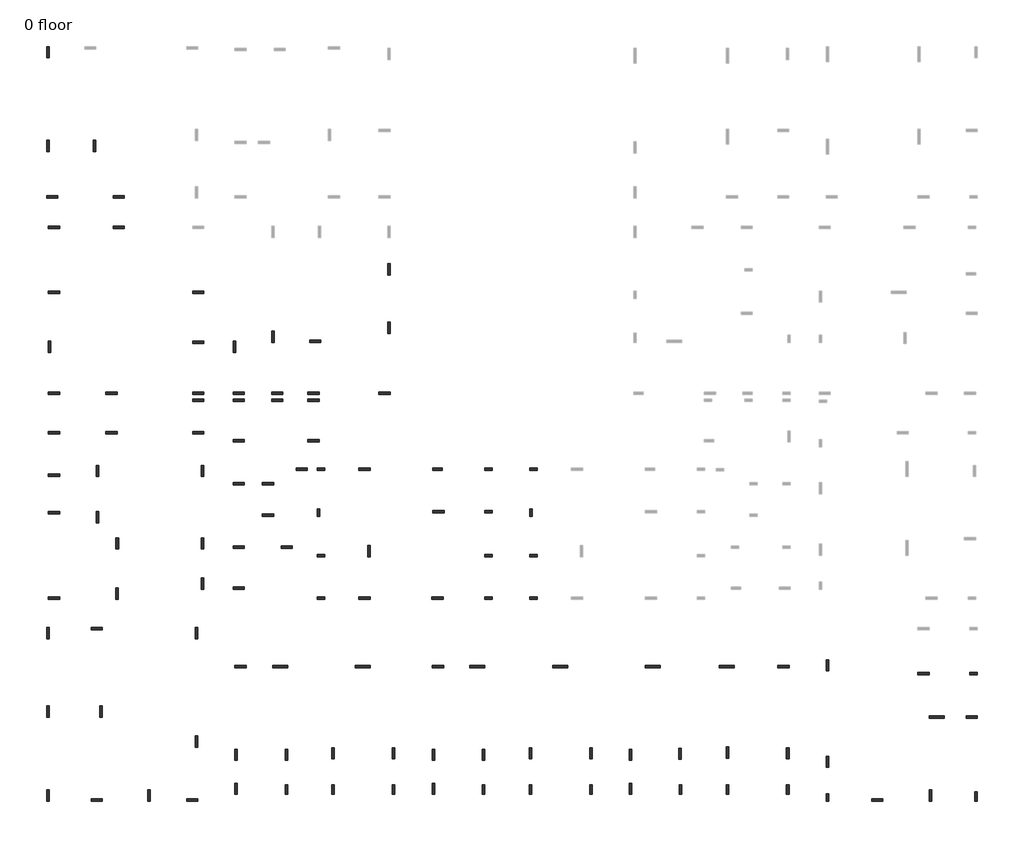
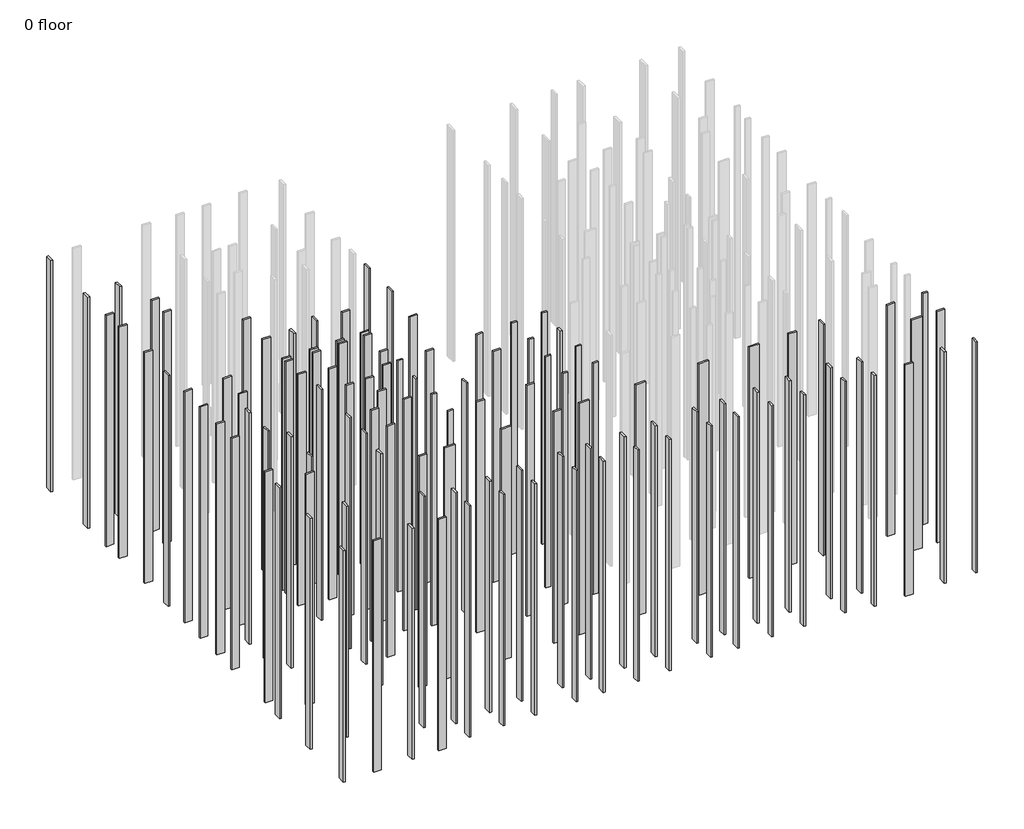
# One storey, part 1 of 2: 120 columns.
"""IFC4 building model written with IfcOpenShell, lengths in millimetres."""

from ifc_helpers import new_model, si_unit, origin, place, context, project, spatial, transform, mapped, element, save
from components import column_6d4d5e46, column_25705251, column_7936e864, column_a28f250a, column_35a9bf28

model = new_model("IFC4")

# Units and contexts
model_context = context("Model", 3, world=origin())
ifc_project = project(units=[si_unit("LENGTHUNIT", "METRE", prefix="MILLI")], contexts=[model_context])

# Site, building, storey
site = spatial("IfcSite", under=ifc_project)
building = spatial("IfcBuilding", under=site)
storey = spatial("IfcBuildingStorey", under=building, Name="0 floor", Elevation=0.0)

# Columns
placement = place(None, origin())
column_shape = column_6d4d5e46(model_context)
element("IfcColumn", 1, ObjectType="Rectangular Column : 2' x 8\"", at=placement, inside=storey, context=model_context, shape_type="MappedRepresentation", body=[
    mapped(column_shape, transform((32806.420549, -1853.4069385, 0.0), x_axis=(1.0, 0.0, 0.0), y_axis=(0.0, 1.0, 0.0), z_axis=(0.0, 0.0, 1.0))),
])
element("IfcColumn", 2, ObjectType="Rectangular Column : 2' x 8\"", at=placement, inside=storey, context=model_context, shape_type="MappedRepresentation", body=[
    mapped(column_shape, transform((20944.620549, -11911.8069385, 0.0), x_axis=(0.0, 1.0, 0.0), y_axis=(-1.0, 0.0, 0.0), z_axis=(0.0, 0.0, 1.0))),
])
element("IfcColumn", 3, ObjectType="Rectangular Column : 2' x 8\"", at=placement, inside=storey, context=model_context, shape_type="MappedRepresentation", body=[
    mapped(column_shape, transform((-20114.479451, 14707.393062, 0.0), x_axis=(1.0, 0.0, 0.0), y_axis=(0.0, 1.0, 0.0), z_axis=(0.0, 0.0, 1.0))),
])
element("IfcColumn", 4, ObjectType="Rectangular Column : 2' x 8\"", at=placement, inside=storey, context=model_context, shape_type="MappedRepresentation", body=[
    mapped(column_shape, transform((-6512.7819406, 14707.393062, 0.0), x_axis=(1.0, 0.0, 0.0), y_axis=(0.0, 1.0, 0.0), z_axis=(0.0, 0.0, 1.0))),
])
element("IfcColumn", 5, ObjectType="Rectangular Column : 2' x 8\"", at=placement, inside=storey, context=model_context, shape_type="MappedRepresentation", body=[
    mapped(column_shape, transform((-6512.779451, 4255.2930586, 0.0), x_axis=(1.0, 0.0, 0.0), y_axis=(0.0, 1.0, 0.0), z_axis=(0.0, 0.0, 1.0))),
])
element("IfcColumn", 6, ObjectType="Rectangular Column : 2' x 8\"", at=placement, inside=storey, context=model_context, shape_type="MappedRepresentation", body=[
    mapped(column_shape, transform((-20114.479451, 4255.2930586, 0.0), x_axis=(1.0, 0.0, 0.0), y_axis=(0.0, 1.0, 0.0), z_axis=(0.0, 0.0, 1.0))),
])
element("IfcColumn", 7, ObjectType="Rectangular Column : 2' x 8\"", at=placement, inside=storey, context=model_context, shape_type="MappedRepresentation", body=[
    mapped(column_shape, transform((-20114.479451, 7709.693062, 0.0), x_axis=(1.0, 0.0, 0.0), y_axis=(0.0, 1.0, 0.0), z_axis=(0.0, 0.0, 1.0))),
])
element("IfcColumn", 8, ObjectType="Rectangular Column : 2' x 8\"", at=placement, inside=storey, context=model_context, shape_type="MappedRepresentation", body=[
    mapped(column_shape, transform((-6512.779451, 7709.693062, 0.0), x_axis=(1.0, 0.0, 0.0), y_axis=(0.0, 1.0, 0.0), z_axis=(0.0, 0.0, 1.0))),
])
element("IfcColumn", 9, ObjectType="Rectangular Column : 2' x 8\"", at=placement, inside=storey, context=model_context, shape_type="MappedRepresentation", body=[
    mapped(column_shape, transform((-6512.779451, 11265.693062, 0.0), x_axis=(1.0, 0.0, 0.0), y_axis=(0.0, 1.0, 0.0), z_axis=(0.0, 0.0, 1.0))),
])
element("IfcColumn", 10, ObjectType="Rectangular Column : 2' x 8\"", at=placement, inside=storey, context=model_context, shape_type="MappedRepresentation", body=[
    mapped(column_shape, transform((-20317.679451, 11189.4930571, 0.0), x_axis=(0.0, 1.0, 0.0), y_axis=(-1.0, 0.0, 0.0), z_axis=(0.0, 0.0, 1.0))),
])
element("IfcColumn", 11, ObjectType="Rectangular Column : 2' x 8\"", at=placement, inside=storey, context=model_context, shape_type="MappedRepresentation", body=[
    mapped(column_shape, transform((-2893.279451, 14707.393062, 0.0), x_axis=(1.0, 0.0, 0.0), y_axis=(0.0, 1.0, 0.0), z_axis=(0.0, 0.0, 1.0))),
])
element("IfcColumn", 12, ObjectType="Rectangular Column : 2' x 8\"", at=placement, inside=storey, context=model_context, shape_type="MappedRepresentation", body=[
    mapped(column_shape, transform((-2893.279451, 4255.2930586, 0.0), x_axis=(1.0, 0.0, 0.0), y_axis=(0.0, 1.0, 0.0), z_axis=(0.0, 0.0, 1.0))),
])
element("IfcColumn", 13, ObjectType="Rectangular Column : 2' x 8\"", at=placement, inside=storey, context=model_context, shape_type="MappedRepresentation", body=[
    mapped(column_shape, transform((-2893.279451, 7709.693062, 0.0), x_axis=(1.0, 0.0, 0.0), y_axis=(0.0, 1.0, 0.0), z_axis=(0.0, 0.0, 1.0))),
])
element("IfcColumn", 14, ObjectType="Rectangular Column : 2' x 8\"", at=placement, inside=storey, context=model_context, shape_type="MappedRepresentation", body=[
    mapped(column_shape, transform((-3096.479451, 11189.4930571, 0.0), x_axis=(0.0, 1.0, 0.0), y_axis=(-1.0, 0.0, 0.0), z_axis=(0.0, 0.0, 1.0))),
])
column_2_shape = column_25705251(model_context)
element("IfcColumn", 15, ObjectType="Rectangular Column : 8\" x 2'6\"", at=placement, inside=storey, context=model_context, shape_type="MappedRepresentation", body=[
    mapped(column_2_shape, transform((-19136.579451, -11276.8077465, 0.0), x_axis=(0.0, 1.0, 0.0), y_axis=(-1.0, 0.0, 0.0), z_axis=(0.0, 0.0, 1.0))),
])
element("IfcColumn", 16, ObjectType="Rectangular Column : 8\" x 2'6\"", at=placement, inside=storey, context=model_context, shape_type="MappedRepresentation", body=[
    mapped(column_2_shape, transform((-22921.179445, -11276.8077465, 0.0), x_axis=(0.0, 1.0, 0.0), y_axis=(-1.0, 0.0, 0.0), z_axis=(0.0, 0.0, 1.0))),
])
element("IfcColumn", 17, ObjectType="Rectangular Column : 8\" x 2'6\"", at=placement, inside=storey, context=model_context, shape_type="MappedRepresentation", body=[
    mapped(column_2_shape, transform((-14234.3794399, -11276.807746, 0.0), x_axis=(0.0, 1.0, 0.0), y_axis=(-1.0, 0.0, 0.0), z_axis=(0.0, 0.0, 1.0))),
])
element("IfcColumn", 18, ObjectType="Rectangular Column : 8\" x 2'6\"", at=placement, inside=storey, context=model_context, shape_type="MappedRepresentation", body=[
    mapped(column_2_shape, transform((-3134.5794514, -11276.8077465, 0.0), x_axis=(0.0, 1.0, 0.0), y_axis=(-1.0, 0.0, 0.0), z_axis=(0.0, 0.0, 1.0))),
])
element("IfcColumn", 19, ObjectType="Rectangular Column : 8\" x 2'6\"", at=placement, inside=storey, context=model_context, shape_type="MappedRepresentation", body=[
    mapped(column_2_shape, transform((-6919.1794428, -11276.806938, 0.0), x_axis=(0.0, 1.0, 0.0), y_axis=(-1.0, 0.0, 0.0), z_axis=(0.0, 0.0, 1.0))),
])
element("IfcColumn", 20, ObjectType="Rectangular Column : 8\" x 2'6\"", at=placement, inside=storey, context=model_context, shape_type="MappedRepresentation", body=[
    mapped(column_2_shape, transform((1767.62056, -11276.8077465, 0.0), x_axis=(0.0, 1.0, 0.0), y_axis=(-1.0, 0.0, 0.0), z_axis=(0.0, 0.0, 1.0))),
])
element("IfcColumn", 21, ObjectType="Rectangular Column : 8\" x 2'6\"", at=placement, inside=storey, context=model_context, shape_type="MappedRepresentation", body=[
    mapped(column_2_shape, transform((9044.7230497, -11276.806938, 0.0), x_axis=(0.0, 1.0, 0.0), y_axis=(-1.0, 0.0, 0.0), z_axis=(0.0, 0.0, 1.0))),
])
element("IfcColumn", 22, ObjectType="Rectangular Column : 8\" x 2'6\"", at=placement, inside=storey, context=model_context, shape_type="MappedRepresentation", body=[
    mapped(column_2_shape, transform((12866.8328033, -11276.8077465, 0.0), x_axis=(0.0, 1.0, 0.0), y_axis=(-1.0, 0.0, 0.0), z_axis=(0.0, 0.0, 1.0))),
])
element("IfcColumn", 23, ObjectType="Rectangular Column : 8\" x 2'6\"", at=placement, inside=storey, context=model_context, shape_type="MappedRepresentation", body=[
    mapped(column_2_shape, transform((17731.5205605, -11276.807746, 0.0), x_axis=(0.0, 1.0, 0.0), y_axis=(-1.0, 0.0, 0.0), z_axis=(0.0, 0.0, 1.0))),
])
element("IfcColumn", 24, ObjectType="Rectangular Column : 8\" x 2'6\"", at=placement, inside=storey, context=model_context, shape_type="MappedRepresentation", body=[
    mapped(column_2_shape, transform((33009.620549, -11835.6069385, 0.0), x_axis=(0.0, 1.0, 0.0), y_axis=(-1.0, 0.0, 0.0), z_axis=(0.0, 0.0, 1.0))),
])
element("IfcColumn", 25, ObjectType="Rectangular Column : 8\" x 2'6\"", at=placement, inside=storey, context=model_context, shape_type="MappedRepresentation", body=[
    mapped(column_2_shape, transform((-10652.979451, 14707.393062, 0.0), x_axis=(1.0, 0.0, 0.0), y_axis=(0.0, 1.0, 0.0), z_axis=(0.0, 0.0, 1.0))),
])
column_3_shape = column_7936e864(model_context)
element("IfcColumn", 26, ObjectType="Rectangular Column : 8\" x 3'", at=placement, inside=storey, context=model_context, shape_type="MappedRepresentation", body=[
    mapped(column_3_shape, transform((-42257.4159199, 48540.1930552, 0.0), x_axis=(0.0, 1.0, 0.0), y_axis=(-1.0, 0.0, 0.0), z_axis=(0.0, 0.0, 1.0))),
])
element("IfcColumn", 27, ObjectType="Rectangular Column : 8\" x 3'", at=placement, inside=storey, context=model_context, shape_type="MappedRepresentation", body=[
    mapped(column_3_shape, transform((-42257.4159175, 40932.8930553, 0.0), x_axis=(0.0, 1.0, 0.0), y_axis=(-1.0, 0.0, 0.0), z_axis=(0.0, 0.0, 1.0))),
])
element("IfcColumn", 28, ObjectType="Rectangular Column : 8\" x 3'", at=placement, inside=storey, context=model_context, shape_type="MappedRepresentation", body=[
    mapped(column_3_shape, transform((-38457.2844598, 40932.8930585, 0.0), x_axis=(0.0, 1.0, 0.0), y_axis=(-1.0, 0.0, 0.0), z_axis=(0.0, 0.0, 1.0))),
])
element("IfcColumn", 29, ObjectType="Rectangular Column : 8\" x 3'", at=placement, inside=storey, context=model_context, shape_type="MappedRepresentation", body=[
    mapped(column_3_shape, transform((-41901.8159175, 36805.393059, 0.0), x_axis=(-1.0, 0.0, 0.0), y_axis=(0.0, -1.0, 0.0), z_axis=(0.0, 0.0, 1.0))),
])
element("IfcColumn", 30, ObjectType="Rectangular Column : 8\" x 3'", at=placement, inside=storey, context=model_context, shape_type="MappedRepresentation", body=[
    mapped(column_3_shape, transform((-36500.310909, 36805.393059, 0.0), x_axis=(-1.0, 0.0, 0.0), y_axis=(0.0, -1.0, 0.0), z_axis=(0.0, 0.0, 1.0))),
])
element("IfcColumn", 31, ObjectType="Rectangular Column : 8\" x 3'", at=placement, inside=storey, context=model_context, shape_type="MappedRepresentation", body=[
    mapped(column_3_shape, transform((-41758.110909, 34316.193061, 0.0), x_axis=(1.0, 0.0, 0.0), y_axis=(0.0, 1.0, 0.0), z_axis=(0.0, 0.0, 1.0))),
])
element("IfcColumn", 32, ObjectType="Rectangular Column : 8\" x 3'", at=placement, inside=storey, context=model_context, shape_type="MappedRepresentation", body=[
    mapped(column_3_shape, transform((-36500.310909, 34316.193059, 0.0), x_axis=(1.0, 0.0, 0.0), y_axis=(0.0, 1.0, 0.0), z_axis=(0.0, 0.0, 1.0))),
])
element("IfcColumn", 33, ObjectType="Rectangular Column : 8\" x 3'", at=placement, inside=storey, context=model_context, shape_type="MappedRepresentation", body=[
    mapped(column_3_shape, transform((-30058.579451, 29071.0930594, 0.0), x_axis=(1.0, 0.0, 0.0), y_axis=(0.0, 1.0, 0.0), z_axis=(0.0, 0.0, 1.0))),
])
element("IfcColumn", 34, ObjectType="Rectangular Column : 8\" x 3'", at=placement, inside=storey, context=model_context, shape_type="MappedRepresentation", body=[
    mapped(column_3_shape, transform((-41758.110909, 29071.0930594, 0.0), x_axis=(1.0, 0.0, 0.0), y_axis=(0.0, 1.0, 0.0), z_axis=(0.0, 0.0, 1.0))),
])
element("IfcColumn", 35, ObjectType="Rectangular Column : 8\" x 3'", at=placement, inside=storey, context=model_context, shape_type="MappedRepresentation", body=[
    mapped(column_3_shape, transform((-42113.7109116, 24641.6245258, 0.0), x_axis=(0.0, 1.0, 0.0), y_axis=(-1.0, 0.0, 0.0), z_axis=(0.0, 0.0, 1.0))),
])
element("IfcColumn", 36, ObjectType="Rectangular Column : 8\" x 3'", at=placement, inside=storey, context=model_context, shape_type="MappedRepresentation", body=[
    mapped(column_3_shape, transform((-37084.510909, 20892.2930585, 0.0), x_axis=(-1.0, 0.0, 0.0), y_axis=(0.0, -1.0, 0.0), z_axis=(0.0, 0.0, 1.0))),
])
element("IfcColumn", 37, ObjectType="Rectangular Column : 8\" x 3'", at=placement, inside=storey, context=model_context, shape_type="MappedRepresentation", body=[
    mapped(column_3_shape, transform((-41755.2794479, 20892.2930585, 0.0), x_axis=(-1.0, 0.0, 0.0), y_axis=(0.0, -1.0, 0.0), z_axis=(0.0, 0.0, 1.0))),
])
element("IfcColumn", 38, ObjectType="Rectangular Column : 8\" x 3'", at=placement, inside=storey, context=model_context, shape_type="MappedRepresentation", body=[
    mapped(column_3_shape, transform((-14612.3473752, 30925.2930587, 0.0), x_axis=(0.0, -1.0, 0.0), y_axis=(1.0, 0.0, 0.0), z_axis=(0.0, 0.0, 1.0))),
])
element("IfcColumn", 39, ObjectType="Rectangular Column : 8\" x 3'", at=placement, inside=storey, context=model_context, shape_type="MappedRepresentation", body=[
    mapped(column_3_shape, transform((-14612.3473752, 26175.4930592, 0.0), x_axis=(0.0, -1.0, 0.0), y_axis=(1.0, 0.0, 0.0), z_axis=(0.0, 0.0, 1.0))),
])
element("IfcColumn", 40, ObjectType="Rectangular Column : 8\" x 3'", at=placement, inside=storey, context=model_context, shape_type="MappedRepresentation", body=[
    mapped(column_3_shape, transform((-27134.5473751, 24651.493059, 0.0), x_axis=(0.0, -1.0, 0.0), y_axis=(1.0, 0.0, 0.0), z_axis=(0.0, 0.0, 1.0))),
])
element("IfcColumn", 41, ObjectType="Rectangular Column : 8\" x 3'", at=placement, inside=storey, context=model_context, shape_type="MappedRepresentation", body=[
    mapped(column_3_shape, transform((-24010.3473751, 25464.293061, 0.0), x_axis=(0.0, -1.0, 0.0), y_axis=(1.0, 0.0, 0.0), z_axis=(0.0, 0.0, 1.0))),
])
element("IfcColumn", 42, ObjectType="Rectangular Column : 8\" x 3'", at=placement, inside=storey, context=model_context, shape_type="MappedRepresentation", body=[
    mapped(column_3_shape, transform((-20568.647375, 25108.6930594, 0.0), x_axis=(1.0, 0.0, 0.0), y_axis=(0.0, 1.0, 0.0), z_axis=(0.0, 0.0, 1.0))),
])
element("IfcColumn", 43, ObjectType="Rectangular Column : 8\" x 3'", at=placement, inside=storey, context=model_context, shape_type="MappedRepresentation", body=[
    mapped(column_3_shape, transform((-20718.2159173, 20892.2930592, 0.0), x_axis=(1.0, 0.0, 0.0), y_axis=(0.0, 1.0, 0.0), z_axis=(0.0, 0.0, 1.0))),
])
element("IfcColumn", 44, ObjectType="Rectangular Column : 8\" x 3'", at=placement, inside=storey, context=model_context, shape_type="MappedRepresentation", body=[
    mapped(column_3_shape, transform((-20718.2159173, 20308.0930621, 0.0), x_axis=(1.0, 0.0, 0.0), y_axis=(0.0, 1.0, 0.0), z_axis=(0.0, 0.0, 1.0))),
])
element("IfcColumn", 45, ObjectType="Rectangular Column : 8\" x 3'", at=placement, inside=storey, context=model_context, shape_type="MappedRepresentation", body=[
    mapped(column_3_shape, transform((-23654.7473751, 20892.2930592, 0.0), x_axis=(1.0, 0.0, 0.0), y_axis=(0.0, 1.0, 0.0), z_axis=(0.0, 0.0, 1.0))),
])
element("IfcColumn", 46, ObjectType="Rectangular Column : 8\" x 3'", at=placement, inside=storey, context=model_context, shape_type="MappedRepresentation", body=[
    mapped(column_3_shape, transform((-23654.7473751, 20308.0930621, 0.0), x_axis=(1.0, 0.0, 0.0), y_axis=(0.0, 1.0, 0.0), z_axis=(0.0, 0.0, 1.0))),
])
element("IfcColumn", 47, ObjectType="Rectangular Column : 8\" x 3'", at=placement, inside=storey, context=model_context, shape_type="MappedRepresentation", body=[
    mapped(column_3_shape, transform((-26776.1159173, 20892.2930592, 0.0), x_axis=(1.0, 0.0, 0.0), y_axis=(0.0, 1.0, 0.0), z_axis=(0.0, 0.0, 1.0))),
])
element("IfcColumn", 48, ObjectType="Rectangular Column : 8\" x 3'", at=placement, inside=storey, context=model_context, shape_type="MappedRepresentation", body=[
    mapped(column_3_shape, transform((-26776.1159173, 20308.093062, 0.0), x_axis=(1.0, 0.0, 0.0), y_axis=(0.0, 1.0, 0.0), z_axis=(0.0, 0.0, 1.0))),
])
element("IfcColumn", 49, ObjectType="Rectangular Column : 8\" x 3'", at=placement, inside=storey, context=model_context, shape_type="MappedRepresentation", body=[
    mapped(column_3_shape, transform((-14967.9473752, 20892.2930592, 0.0), x_axis=(1.0, 0.0, 0.0), y_axis=(0.0, 1.0, 0.0), z_axis=(0.0, 0.0, 1.0))),
])
element("IfcColumn", 50, ObjectType="Rectangular Column : 8\" x 3'", at=placement, inside=storey, context=model_context, shape_type="MappedRepresentation", body=[
    mapped(column_3_shape, transform((-30058.579451, 25007.093059, 0.0), x_axis=(1.0, 0.0, 0.0), y_axis=(0.0, 1.0, 0.0), z_axis=(0.0, 0.0, 1.0))),
])
element("IfcColumn", 51, ObjectType="Rectangular Column : 8\" x 3'", at=placement, inside=storey, context=model_context, shape_type="MappedRepresentation", body=[
    mapped(column_3_shape, transform((-30058.579451, 20892.2930585, 0.0), x_axis=(1.0, 0.0, 0.0), y_axis=(0.0, 1.0, 0.0), z_axis=(0.0, 0.0, 1.0))),
])
element("IfcColumn", 52, ObjectType="Rectangular Column : 8\" x 3'", at=placement, inside=storey, context=model_context, shape_type="MappedRepresentation", body=[
    mapped(column_3_shape, transform((-30058.579451, 20308.0930613, 0.0), x_axis=(1.0, 0.0, 0.0), y_axis=(0.0, 1.0, 0.0), z_axis=(0.0, 0.0, 1.0))),
])
element("IfcColumn", 53, ObjectType="Rectangular Column : 8\" x 3'", at=placement, inside=storey, context=model_context, shape_type="MappedRepresentation", body=[
    mapped(column_3_shape, transform((-30058.579451, 17679.1930621, 0.0), x_axis=(1.0, 0.0, 0.0), y_axis=(0.0, 1.0, 0.0), z_axis=(0.0, 0.0, 1.0))),
])
element("IfcColumn", 54, ObjectType="Rectangular Column : 8\" x 3'", at=placement, inside=storey, context=model_context, shape_type="MappedRepresentation", body=[
    mapped(column_3_shape, transform((-29705.3114637, 14580.3930626, 0.0), x_axis=(0.0, 1.0, 0.0), y_axis=(-1.0, 0.0, 0.0), z_axis=(0.0, 0.0, 1.0))),
])
element("IfcColumn", 55, ObjectType="Rectangular Column : 8\" x 3'", at=placement, inside=storey, context=model_context, shape_type="MappedRepresentation", body=[
    mapped(column_3_shape, transform((-29705.3114638, 8687.5930659, 0.0), x_axis=(0.0, 1.0, 0.0), y_axis=(-1.0, 0.0, 0.0), z_axis=(0.0, 0.0, 1.0))),
])
element("IfcColumn", 56, ObjectType="Rectangular Column : 8\" x 3'", at=placement, inside=storey, context=model_context, shape_type="MappedRepresentation", body=[
    mapped(column_3_shape, transform((-29702.979451, 5436.3930634, 0.0), x_axis=(0.0, 1.0, 0.0), y_axis=(-1.0, 0.0, 0.0), z_axis=(0.0, 0.0, 1.0))),
])
element("IfcColumn", 57, ObjectType="Rectangular Column : 8\" x 3'", at=placement, inside=storey, context=model_context, shape_type="MappedRepresentation", body=[
    mapped(column_3_shape, transform((-26776.1159173, 5080.7930617, 0.0), x_axis=(-1.0, 0.0, 0.0), y_axis=(0.0, -1.0, 0.0), z_axis=(0.0, 0.0, 1.0))),
])
element("IfcColumn", 58, ObjectType="Rectangular Column : 8\" x 3'", at=placement, inside=storey, context=model_context, shape_type="MappedRepresentation", body=[
    mapped(column_3_shape, transform((-26776.1159173, 8382.7930618, 0.0), x_axis=(-1.0, 0.0, 0.0), y_axis=(0.0, -1.0, 0.0), z_axis=(0.0, 0.0, 1.0))),
])
element("IfcColumn", 59, ObjectType="Rectangular Column : 8\" x 3'", at=placement, inside=storey, context=model_context, shape_type="MappedRepresentation", body=[
    mapped(column_3_shape, transform((-24413.9159173, 10973.5930617, 0.0), x_axis=(-1.0, 0.0, 0.0), y_axis=(0.0, -1.0, 0.0), z_axis=(0.0, 0.0, 1.0))),
])
element("IfcColumn", 60, ObjectType="Rectangular Column : 8\" x 3'", at=placement, inside=storey, context=model_context, shape_type="MappedRepresentation", body=[
    mapped(column_3_shape, transform((-22889.9159173, 8382.7930618, 0.0), x_axis=(-1.0, 0.0, 0.0), y_axis=(0.0, -1.0, 0.0), z_axis=(0.0, 0.0, 1.0))),
])
element("IfcColumn", 61, ObjectType="Rectangular Column : 8\" x 3'", at=placement, inside=storey, context=model_context, shape_type="MappedRepresentation", body=[
    mapped(column_3_shape, transform((-41755.2794479, 17679.1930621, 0.0), x_axis=(-1.0, 0.0, 0.0), y_axis=(0.0, -1.0, 0.0), z_axis=(0.0, 0.0, 1.0))),
])
element("IfcColumn", 62, ObjectType="Rectangular Column : 8\" x 3'", at=placement, inside=storey, context=model_context, shape_type="MappedRepresentation", body=[
    mapped(column_3_shape, transform((-37084.510909, 17679.1930621, 0.0), x_axis=(-1.0, 0.0, 0.0), y_axis=(0.0, -1.0, 0.0), z_axis=(0.0, 0.0, 1.0))),
])
element("IfcColumn", 63, ObjectType="Rectangular Column : 8\" x 3'", at=placement, inside=storey, context=model_context, shape_type="MappedRepresentation", body=[
    mapped(column_3_shape, transform((-41755.2794479, 14224.7930621, 0.0), x_axis=(-1.0, 0.0, 0.0), y_axis=(0.0, -1.0, 0.0), z_axis=(0.0, 0.0, 1.0))),
])
element("IfcColumn", 64, ObjectType="Rectangular Column : 8\" x 3'", at=placement, inside=storey, context=model_context, shape_type="MappedRepresentation", body=[
    mapped(column_3_shape, transform((-38237.379451, 14580.3930621, 0.0), x_axis=(0.0, -1.0, 0.0), y_axis=(1.0, 0.0, 0.0), z_axis=(0.0, 0.0, 1.0))),
])
element("IfcColumn", 65, ObjectType="Rectangular Column : 8\" x 3'", at=placement, inside=storey, context=model_context, shape_type="MappedRepresentation", body=[
    mapped(column_3_shape, transform((-41755.279451, 11176.7930621, 0.0), x_axis=(1.0, 0.0, 0.0), y_axis=(0.0, 1.0, 0.0), z_axis=(0.0, 0.0, 1.0))),
])
element("IfcColumn", 66, ObjectType="Rectangular Column : 8\" x 3'", at=placement, inside=storey, context=model_context, shape_type="MappedRepresentation", body=[
    mapped(column_3_shape, transform((-38237.379451, 10821.1930653, 0.0), x_axis=(0.0, 1.0, 0.0), y_axis=(-1.0, 0.0, 0.0), z_axis=(0.0, 0.0, 1.0))),
])
element("IfcColumn", 67, ObjectType="Rectangular Column : 8\" x 3'", at=placement, inside=storey, context=model_context, shape_type="MappedRepresentation", body=[
    mapped(column_3_shape, transform((-36649.879451, 4610.8930621, 0.0), x_axis=(0.0, 1.0, 0.0), y_axis=(-1.0, 0.0, 0.0), z_axis=(0.0, 0.0, 1.0))),
])
element("IfcColumn", 68, ObjectType="Rectangular Column : 8\" x 3'", at=placement, inside=storey, context=model_context, shape_type="MappedRepresentation", body=[
    mapped(column_3_shape, transform((-41755.2794511, 4255.2930621, 0.0), x_axis=(-1.0, 0.0, 0.0), y_axis=(0.0, -1.0, 0.0), z_axis=(0.0, 0.0, 1.0))),
])
element("IfcColumn", 69, ObjectType="Rectangular Column : 8\" x 3'", at=placement, inside=storey, context=model_context, shape_type="MappedRepresentation", body=[
    mapped(column_3_shape, transform((-38288.179451, 1766.0930615, 0.0), x_axis=(-1.0, 0.0, 0.0), y_axis=(0.0, -1.0, 0.0), z_axis=(0.0, 0.0, 1.0))),
])
element("IfcColumn", 70, ObjectType="Rectangular Column : 8\" x 3'", at=placement, inside=storey, context=model_context, shape_type="MappedRepresentation", body=[
    mapped(column_3_shape, transform((-42257.4159175, 1410.4930647, 0.0), x_axis=(0.0, -1.0, 0.0), y_axis=(1.0, 0.0, 0.0), z_axis=(0.0, 0.0, 1.0))),
])
element("IfcColumn", 71, ObjectType="Rectangular Column : 8\" x 3'", at=placement, inside=storey, context=model_context, shape_type="MappedRepresentation", body=[
    mapped(column_3_shape, transform((-30198.279451, 1410.4930647, 0.0), x_axis=(0.0, -1.0, 0.0), y_axis=(1.0, 0.0, 0.0), z_axis=(0.0, 0.0, 1.0))),
])
element("IfcColumn", 72, ObjectType="Rectangular Column : 8\" x 3'", at=placement, inside=storey, context=model_context, shape_type="MappedRepresentation", body=[
    mapped(column_3_shape, transform((-37932.579451, -4952.2069385, 0.0), x_axis=(0.0, -1.0, 0.0), y_axis=(1.0, 0.0, 0.0), z_axis=(0.0, 0.0, 1.0))),
])
element("IfcColumn", 73, ObjectType="Rectangular Column : 8\" x 3'", at=placement, inside=storey, context=model_context, shape_type="MappedRepresentation", body=[
    mapped(column_3_shape, transform((-42257.4159144, -4952.2069385, 0.0), x_axis=(0.0, -1.0, 0.0), y_axis=(1.0, 0.0, 0.0), z_axis=(0.0, 0.0, 1.0))),
])
element("IfcColumn", 74, ObjectType="Rectangular Column : 8\" x 3'", at=placement, inside=storey, context=model_context, shape_type="MappedRepresentation", body=[
    mapped(column_3_shape, transform((-42257.4159175, -11759.4069385, 0.0), x_axis=(0.0, -1.0, 0.0), y_axis=(1.0, 0.0, 0.0), z_axis=(0.0, 0.0, 1.0))),
])
element("IfcColumn", 75, ObjectType="Rectangular Column : 8\" x 3'", at=placement, inside=storey, context=model_context, shape_type="MappedRepresentation", body=[
    mapped(column_3_shape, transform((-38288.179451, -12115.0069385, 0.0), x_axis=(1.0, 0.0, 0.0), y_axis=(0.0, 1.0, 0.0), z_axis=(0.0, 0.0, 1.0))),
])
element("IfcColumn", 76, ObjectType="Rectangular Column : 8\" x 3'", at=placement, inside=storey, context=model_context, shape_type="MappedRepresentation", body=[
    mapped(column_3_shape, transform((-34059.079451, -11759.4069384, 0.0), x_axis=(0.0, 1.0, 0.0), y_axis=(-1.0, 0.0, 0.0), z_axis=(0.0, 0.0, 1.0))),
])
element("IfcColumn", 77, ObjectType="Rectangular Column : 8\" x 3'", at=placement, inside=storey, context=model_context, shape_type="MappedRepresentation", body=[
    mapped(column_3_shape, transform((-30553.8794481, -12115.0069385, 0.0), x_axis=(-1.0, 0.0, 0.0), y_axis=(0.0, -1.0, 0.0), z_axis=(0.0, 0.0, 1.0))),
])
element("IfcColumn", 78, ObjectType="Rectangular Column : 8\" x 3'", at=placement, inside=storey, context=model_context, shape_type="MappedRepresentation", body=[
    mapped(column_3_shape, transform((-30198.279451, -7377.9069383, 0.0), x_axis=(0.0, -1.0, 0.0), y_axis=(1.0, 0.0, 0.0), z_axis=(0.0, 0.0, 1.0))),
])
element("IfcColumn", 79, ObjectType="Rectangular Column : 8\" x 3'", at=placement, inside=storey, context=model_context, shape_type="MappedRepresentation", body=[
    mapped(column_3_shape, transform((-26776.1159173, 17006.0930621, 0.0), x_axis=(1.0, 0.0, 0.0), y_axis=(0.0, 1.0, 0.0), z_axis=(0.0, 0.0, 1.0))),
])
element("IfcColumn", 80, ObjectType="Rectangular Column : 8\" x 3'", at=placement, inside=storey, context=model_context, shape_type="MappedRepresentation", body=[
    mapped(column_3_shape, transform((-20718.2159173, 17006.0930621, 0.0), x_axis=(1.0, 0.0, 0.0), y_axis=(0.0, 1.0, 0.0), z_axis=(0.0, 0.0, 1.0))),
])
element("IfcColumn", 81, ObjectType="Rectangular Column : 8\" x 3'", at=placement, inside=storey, context=model_context, shape_type="MappedRepresentation", body=[
    mapped(column_3_shape, transform((-21670.7159173, 14707.3930651, 0.0), x_axis=(1.0, 0.0, 0.0), y_axis=(0.0, 1.0, 0.0), z_axis=(0.0, 0.0, 1.0))),
])
element("IfcColumn", 82, ObjectType="Rectangular Column : 8\" x 3'", at=placement, inside=storey, context=model_context, shape_type="MappedRepresentation", body=[
    mapped(column_3_shape, transform((-24413.9159173, 13538.9930617, 0.0), x_axis=(1.0, 0.0, 0.0), y_axis=(0.0, 1.0, 0.0), z_axis=(0.0, 0.0, 1.0))),
])
element("IfcColumn", 83, ObjectType="Rectangular Column : 8\" x 3'", at=placement, inside=storey, context=model_context, shape_type="MappedRepresentation", body=[
    mapped(column_3_shape, transform((-26776.1159175, 13538.9930617, 0.0), x_axis=(1.0, 0.0, 0.0), y_axis=(0.0, 1.0, 0.0), z_axis=(0.0, 0.0, 1.0))),
])
element("IfcColumn", 84, ObjectType="Rectangular Column : 8\" x 3'", at=placement, inside=storey, context=model_context, shape_type="MappedRepresentation", body=[
    mapped(column_3_shape, transform((-26985.1794514, -11200.607746, 0.0), x_axis=(0.0, 1.0, 0.0), y_axis=(-1.0, 0.0, 0.0), z_axis=(0.0, 0.0, 1.0))),
])
element("IfcColumn", 85, ObjectType="Rectangular Column : 8\" x 3'", at=placement, inside=storey, context=model_context, shape_type="MappedRepresentation", body=[
    mapped(column_3_shape, transform((-26985.179451, -8457.407744, 0.0), x_axis=(0.0, 1.0, 0.0), y_axis=(-1.0, 0.0, 0.0), z_axis=(0.0, 0.0, 1.0))),
])
element("IfcColumn", 86, ObjectType="Rectangular Column : 8\" x 3'", at=placement, inside=storey, context=model_context, shape_type="MappedRepresentation", body=[
    mapped(column_3_shape, transform((-26629.5794514, -1281.906938, 0.0), x_axis=(1.0, 0.0, 0.0), y_axis=(0.0, 1.0, 0.0), z_axis=(0.0, 0.0, 1.0))),
])
element("IfcColumn", 87, ObjectType="Rectangular Column : 8\" x 3'", at=placement, inside=storey, context=model_context, shape_type="MappedRepresentation", body=[
    mapped(column_3_shape, transform((-22921.179445, -8457.407743, 0.0), x_axis=(0.0, 1.0, 0.0), y_axis=(-1.0, 0.0, 0.0), z_axis=(0.0, 0.0, 1.0))),
])
element("IfcColumn", 88, ObjectType="Rectangular Column : 8\" x 3'", at=placement, inside=storey, context=model_context, shape_type="MappedRepresentation", body=[
    mapped(column_3_shape, transform((-19136.579451, -8330.406938, 0.0), x_axis=(0.0, 1.0, 0.0), y_axis=(-1.0, 0.0, 0.0), z_axis=(0.0, 0.0, 1.0))),
])
element("IfcColumn", 89, ObjectType="Rectangular Column : 8\" x 3'", at=placement, inside=storey, context=model_context, shape_type="MappedRepresentation", body=[
    mapped(column_3_shape, transform((-14234.379451, -8330.406938, 0.0), x_axis=(0.0, 1.0, 0.0), y_axis=(-1.0, 0.0, 0.0), z_axis=(0.0, 0.0, 1.0))),
])
element("IfcColumn", 90, ObjectType="Rectangular Column : 8\" x 3'", at=placement, inside=storey, context=model_context, shape_type="MappedRepresentation", body=[
    mapped(column_3_shape, transform((-10983.179451, -8457.407744, 0.0), x_axis=(0.0, 1.0, 0.0), y_axis=(-1.0, 0.0, 0.0), z_axis=(0.0, 0.0, 1.0))),
])
element("IfcColumn", 91, ObjectType="Rectangular Column : 8\" x 3'", at=placement, inside=storey, context=model_context, shape_type="MappedRepresentation", body=[
    mapped(column_3_shape, transform((-10983.179451, -11200.607746, 0.0), x_axis=(0.0, 1.0, 0.0), y_axis=(-1.0, 0.0, 0.0), z_axis=(0.0, 0.0, 1.0))),
])
element("IfcColumn", 92, ObjectType="Rectangular Column : 8\" x 3'", at=placement, inside=storey, context=model_context, shape_type="MappedRepresentation", body=[
    mapped(column_3_shape, transform((-6919.1794428, -8457.407743, 0.0), x_axis=(0.0, 1.0, 0.0), y_axis=(-1.0, 0.0, 0.0), z_axis=(0.0, 0.0, 1.0))),
])
element("IfcColumn", 93, ObjectType="Rectangular Column : 8\" x 3'", at=placement, inside=storey, context=model_context, shape_type="MappedRepresentation", body=[
    mapped(column_3_shape, transform((-3134.579451, -8330.406938, 0.0), x_axis=(0.0, 1.0, 0.0), y_axis=(-1.0, 0.0, 0.0), z_axis=(0.0, 0.0, 1.0))),
])
element("IfcColumn", 94, ObjectType="Rectangular Column : 8\" x 3'", at=placement, inside=storey, context=model_context, shape_type="MappedRepresentation", body=[
    mapped(column_3_shape, transform((-10627.579451, -1281.906938, 0.0), x_axis=(-1.0, 0.0, 0.0), y_axis=(0.0, -1.0, 0.0), z_axis=(0.0, 0.0, 1.0))),
])
element("IfcColumn", 95, ObjectType="Rectangular Column : 8\" x 3'", at=placement, inside=storey, context=model_context, shape_type="MappedRepresentation", body=[
    mapped(column_3_shape, transform((1767.620549, -8330.406938, 0.0), x_axis=(0.0, 1.0, 0.0), y_axis=(-1.0, 0.0, 0.0), z_axis=(0.0, 0.0, 1.0))),
])
element("IfcColumn", 96, ObjectType="Rectangular Column : 8\" x 3'", at=placement, inside=storey, context=model_context, shape_type="MappedRepresentation", body=[
    mapped(column_3_shape, transform((17375.9205494, -1281.906938, 0.0), x_axis=(1.0, 0.0, 0.0), y_axis=(0.0, 1.0, 0.0), z_axis=(0.0, 0.0, 1.0))),
])
element("IfcColumn", 97, ObjectType="Rectangular Column : 8\" x 3'", at=placement, inside=storey, context=model_context, shape_type="MappedRepresentation", body=[
    mapped(column_3_shape, transform((12841.9479104, -8278.0520526, 0.0), x_axis=(0.0, 1.0, 0.0), y_axis=(-1.0, 0.0, 0.0), z_axis=(0.0, 0.0, 1.0))),
])
element("IfcColumn", 98, ObjectType="Rectangular Column : 8\" x 3'", at=placement, inside=storey, context=model_context, shape_type="MappedRepresentation", body=[
    mapped(column_3_shape, transform((8980.5757278, -8374.0331191, 0.0), x_axis=(0.0, 1.0, 0.0), y_axis=(-1.0, 0.0, 0.0), z_axis=(0.0, 0.0, 1.0))),
])
element("IfcColumn", 99, ObjectType="Rectangular Column : 8\" x 3'", at=placement, inside=storey, context=model_context, shape_type="MappedRepresentation", body=[
    mapped(column_3_shape, transform((17731.5205494, -8330.406938, 0.0), x_axis=(0.0, 1.0, 0.0), y_axis=(-1.0, 0.0, 0.0), z_axis=(0.0, 0.0, 1.0))),
])
element("IfcColumn", 100, ObjectType="Rectangular Column : 8\" x 3'", at=placement, inside=storey, context=model_context, shape_type="MappedRepresentation", body=[
    mapped(column_3_shape, transform((4980.720549, -8457.407744, 0.0), x_axis=(0.0, -1.0, 0.0), y_axis=(1.0, 0.0, 0.0), z_axis=(0.0, 0.0, 1.0))),
])
element("IfcColumn", 101, ObjectType="Rectangular Column : 8\" x 3'", at=placement, inside=storey, context=model_context, shape_type="MappedRepresentation", body=[
    mapped(column_3_shape, transform((4980.720549, -11200.607746, 0.0), x_axis=(0.0, -1.0, 0.0), y_axis=(1.0, 0.0, 0.0), z_axis=(0.0, 0.0, 1.0))),
])
element("IfcColumn", 102, ObjectType="Rectangular Column : 8\" x 3'", at=placement, inside=storey, context=model_context, shape_type="MappedRepresentation", body=[
    mapped(column_3_shape, transform((20944.620549, -9016.2069385, 0.0), x_axis=(0.0, 1.0, 0.0), y_axis=(-1.0, 0.0, 0.0), z_axis=(0.0, 0.0, 1.0))),
])
element("IfcColumn", 103, ObjectType="Rectangular Column : 8\" x 3'", at=placement, inside=storey, context=model_context, shape_type="MappedRepresentation", body=[
    mapped(column_3_shape, transform((24995.920549, -12115.0069385, 0.0), x_axis=(-1.0, 0.0, 0.0), y_axis=(0.0, -1.0, 0.0), z_axis=(0.0, 0.0, 1.0))),
])
element("IfcColumn", 104, ObjectType="Rectangular Column : 8\" x 3'", at=placement, inside=storey, context=model_context, shape_type="MappedRepresentation", body=[
    mapped(column_3_shape, transform((29288.520549, -11759.4069384, 0.0), x_axis=(0.0, -1.0, 0.0), y_axis=(1.0, 0.0, 0.0), z_axis=(0.0, 0.0, 1.0))),
])
element("IfcColumn", 105, ObjectType="Rectangular Column : 8\" x 3'", at=placement, inside=storey, context=model_context, shape_type="MappedRepresentation", body=[
    mapped(column_3_shape, transform((32654.020549, -5409.4069385, 0.0), x_axis=(1.0, 0.0, 0.0), y_axis=(0.0, 1.0, 0.0), z_axis=(0.0, 0.0, 1.0))),
])
element("IfcColumn", 106, ObjectType="Rectangular Column : 8\" x 3'", at=placement, inside=storey, context=model_context, shape_type="MappedRepresentation", body=[
    mapped(column_3_shape, transform((28729.720549, -1853.4069381, 0.0), x_axis=(1.0, 0.0, 0.0), y_axis=(0.0, 1.0, 0.0), z_axis=(0.0, 0.0, 1.0))),
])
element("IfcColumn", 107, ObjectType="Rectangular Column : 8\" x 3'", at=placement, inside=storey, context=model_context, shape_type="MappedRepresentation", body=[
    mapped(column_3_shape, transform((20944.620549, -1193.0069385, 0.0), x_axis=(0.0, 1.0, 0.0), y_axis=(-1.0, 0.0, 0.0), z_axis=(0.0, 0.0, 1.0))),
])
element("IfcColumn", 108, ObjectType="Rectangular Column : 8\" x 3'", at=placement, inside=storey, context=model_context, shape_type="MappedRepresentation", body=[
    mapped(column_3_shape, transform((-10652.979451, 4255.293062, 0.0), x_axis=(1.0, 0.0, 0.0), y_axis=(0.0, 1.0, 0.0), z_axis=(0.0, 0.0, 1.0))),
])
element("IfcColumn", 109, ObjectType="Rectangular Column : 8\" x 3'", at=placement, inside=storey, context=model_context, shape_type="MappedRepresentation", body=[
    mapped(column_3_shape, transform((-16571.179451, 4255.293062, 0.0), x_axis=(1.0, 0.0, 0.0), y_axis=(0.0, 1.0, 0.0), z_axis=(0.0, 0.0, 1.0))),
])
element("IfcColumn", 110, ObjectType="Rectangular Column : 8\" x 3'", at=placement, inside=storey, context=model_context, shape_type="MappedRepresentation", body=[
    mapped(column_3_shape, transform((-16215.579451, 8065.2930636, 0.0), x_axis=(0.0, 1.0, 0.0), y_axis=(-1.0, 0.0, 0.0), z_axis=(0.0, 0.0, 1.0))),
])
element("IfcColumn", 111, ObjectType="Rectangular Column : 8\" x 3'", at=placement, inside=storey, context=model_context, shape_type="MappedRepresentation", body=[
    mapped(column_3_shape, transform((-10573.9479938, 11265.693062, 0.0), x_axis=(-1.0, 0.0, 0.0), y_axis=(0.0, -1.0, 0.0), z_axis=(0.0, 0.0, 1.0))),
])
element("IfcColumn", 112, ObjectType="Rectangular Column : 8\" x 3'", at=placement, inside=storey, context=model_context, shape_type="MappedRepresentation", body=[
    mapped(column_3_shape, transform((-16571.179451, 14707.393062, 0.0), x_axis=(1.0, 0.0, 0.0), y_axis=(0.0, 1.0, 0.0), z_axis=(0.0, 0.0, 1.0))),
])
column_4_shape = column_a28f250a(model_context)
element("IfcColumn", 113, ObjectType="Rectangular Column : 8\" x 4'", at=placement, inside=storey, context=model_context, shape_type="MappedRepresentation", body=[
    mapped(column_4_shape, transform((-23429.1794514, -1281.906938, 0.0), x_axis=(1.0, 0.0, 0.0), y_axis=(0.0, 1.0, 0.0), z_axis=(0.0, 0.0, 1.0))),
])
element("IfcColumn", 114, ObjectType="Rectangular Column : 8\" x 4'", at=placement, inside=storey, context=model_context, shape_type="MappedRepresentation", body=[
    mapped(column_4_shape, transform((-16723.579451, -1281.906938, 0.0), x_axis=(1.0, 0.0, 0.0), y_axis=(0.0, 1.0, 0.0), z_axis=(0.0, 0.0, 1.0))),
])
element("IfcColumn", 115, ObjectType="Rectangular Column : 8\" x 4'", at=placement, inside=storey, context=model_context, shape_type="MappedRepresentation", body=[
    mapped(column_4_shape, transform((-7427.1794511, -1281.906938, 0.0), x_axis=(1.0, 0.0, 0.0), y_axis=(0.0, 1.0, 0.0), z_axis=(0.0, 0.0, 1.0))),
])
element("IfcColumn", 116, ObjectType="Rectangular Column : 8\" x 4'", at=placement, inside=storey, context=model_context, shape_type="MappedRepresentation", body=[
    mapped(column_4_shape, transform((-721.5794506, -1281.906938, 0.0), x_axis=(1.0, 0.0, 0.0), y_axis=(0.0, 1.0, 0.0), z_axis=(0.0, 0.0, 1.0))),
])
element("IfcColumn", 117, ObjectType="Rectangular Column : 8\" x 4'", at=placement, inside=storey, context=model_context, shape_type="MappedRepresentation", body=[
    mapped(column_4_shape, transform((12803.9205601, -1281.906938, 0.0), x_axis=(1.0, 0.0, 0.0), y_axis=(0.0, 1.0, 0.0), z_axis=(0.0, 0.0, 1.0))),
])
element("IfcColumn", 118, ObjectType="Rectangular Column : 8\" x 4'", at=placement, inside=storey, context=model_context, shape_type="MappedRepresentation", body=[
    mapped(column_4_shape, transform((6796.820549, -1281.906938, 0.0), x_axis=(1.0, 0.0, 0.0), y_axis=(0.0, 1.0, 0.0), z_axis=(0.0, 0.0, 1.0))),
])
element("IfcColumn", 119, ObjectType="Rectangular Column : 8\" x 4'", at=placement, inside=storey, context=model_context, shape_type="MappedRepresentation", body=[
    mapped(column_4_shape, transform((29796.520549, -5409.4069385, 0.0), x_axis=(1.0, 0.0, 0.0), y_axis=(0.0, 1.0, 0.0), z_axis=(0.0, 0.0, 1.0))),
])
column_5_shape = column_35a9bf28(model_context)
element("IfcColumn", 120, ObjectType="Rectangular Column : 9\" x 3'", at=placement, inside=storey, context=model_context, shape_type="MappedRepresentation", body=[
    mapped(column_5_shape, transform((-36637.179451, 8687.5930659, 0.0), x_axis=(0.0, 1.0, 0.0), y_axis=(-1.0, 0.0, 0.0), z_axis=(0.0, 0.0, 1.0))),
])

save(model, "model.ifc")

# Revit data of these elements
# Type "Rectangular Column : 2' x 8\""
#   Assembly Code = "B1010200"
#   Depth = 0' - 8"
#   Offset Base = 0' - 0"
#   Offset Top = 0' - 0"
#   Width = 2' - 0"
#   Material = none
# Type "Rectangular Column : 8\" x 2'6\""
#   Assembly Code = "B1010200"
#   Depth = 0' - 8"
#   Offset Base = 0' - 0"
#   Offset Top = 0' - 0"
#   Width = 2' - 6"
#   Material = none
# Type "Rectangular Column : 8\" x 3'"
#   Assembly Code = "B1010200"
#   Depth = 0' - 8"
#   Offset Base = 0' - 0"
#   Offset Top = 0' - 0"
#   Width = 3' - 0"
#   Material = none
# Type "Rectangular Column : 8\" x 4'"
#   Assembly Code = "B1010200"
#   Depth = 0' - 8"
#   Offset Base = 0' - 0"
#   Offset Top = 0' - 0"
#   Width = 4' - 0"
#   Material = none
# Type "Rectangular Column : 9\" x 3'"
#   Assembly Code = "B1010200"
#   Depth = 0' - 9"
#   Offset Base = 0' - 0"
#   Offset Top = 0' - 0"
#   Width = 3' - 0"
#   Material = none
# Elements 1, 2, 3, 4, 5, 6, 7, 8, 9, 10, 11, 12, 13, 14 (IfcColumn, "Rectangular Column : 2' x 8\"")
#   Phase Created = New Construction
# Elements 15, 16, 17, 18, 19, 20, 21, 22, 23, 24, 25 (IfcColumn, "Rectangular Column : 8\" x 2'6\"")
#   Phase Created = New Construction
# Elements 26, 27, 28, 29, 30, 31, 32, 33, 34, 35, 36, 37, 38, 39, 40, 41, 42, 43, 44, 45, 46, 47, 48, 49, 50, 51, 52, 53, 54, 55, 56, 57, 58, 59, 60, 61, 62, 63, 64, 65, 66, 67, 68, 69, 70, 71, 72, 73, 74, 75, 76, 77, 78, 79, 80, 81, 82, 83, 84, 85, 86, 87, 88, 89, 90, 91, 92, 93, 94, 95, 96, 97, 98, 99, 100, 101, 102, 103, 104, 105, 106, 107, 108, 109, 110, 111, 112 (IfcColumn, "Rectangular Column : 8\" x 3'")
#   Phase Created = New Construction
# Elements 113, 114, 115, 116, 117, 118, 119 (IfcColumn, "Rectangular Column : 8\" x 4'")
#   Phase Created = New Construction
# Element 120 (IfcColumn, "Rectangular Column : 9\" x 3'")
#   Phase Created = New Construction
